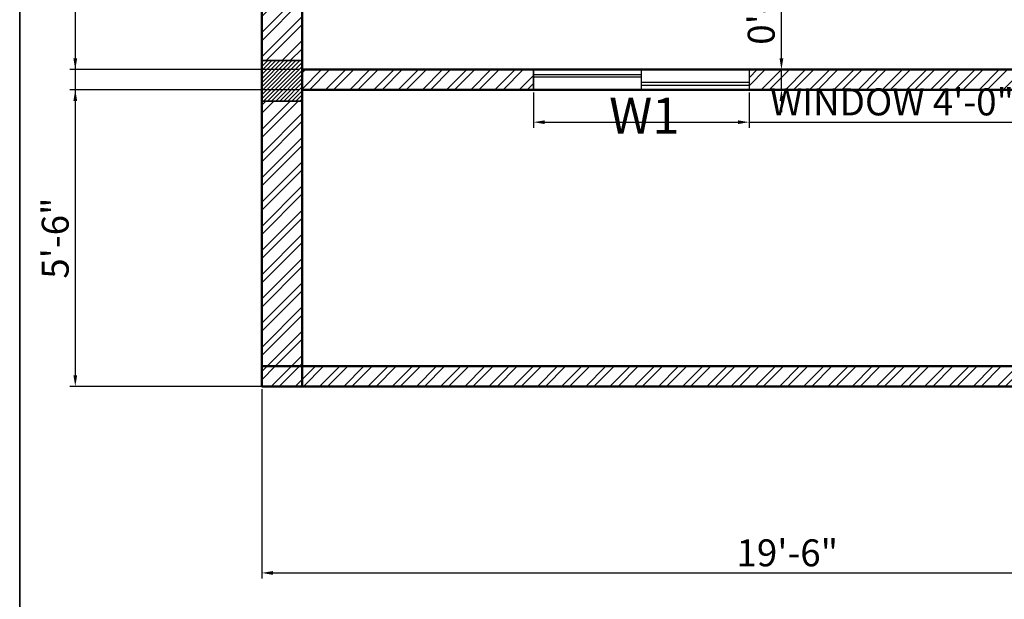
# Model space of a CAD drawing. Units: millimetres. Extents: x 20768 to 23556, y 50760 to 52704.
# Tile 15 of 36: x 21272 to 21491, y 51783 to 51912. Entities that reach past the tile are written whole.
import ezdxf

# ---------------------------------------------------------------- set-up
doc = ezdxf.new("R2010")
doc.units = ezdxf.units.MM
for name, color, linetype, lineweight in [('A-ANNO-TTLB', 7, 'Continuous', 35), ('A-AREA-IDEN', 40, 'Continuous', 18), ('A-GLAZ', 4, 'Continuous', 25), ('A-WALL', 7, 'Continuous', 50), ('A-WALL-PATT', 8, 'Continuous', 13), ('S-ANNO-DIMS', 2, 'Continuous', 18), ('S-COLS', 20, 'Continuous', 35)]:
    doc.layers.add(name, color=color, linetype=linetype, lineweight=lineweight)
doc.styles.get("Standard").update_dxf_attribs({"font": 'arial.ttf'})
doc.dimstyles.new('ISO-25', dxfattribs={"dimtxt": 6, "dimasz": 2.5, "dimexe": 1.25, "dimexo": 0.625, "dimtad": 1, "dimdec": 0, "dimlunit": 3, "dimtxsty": 'Standard', "dimcen": 2.5, "dimadec": 0, "dimazin": 0, "dimtfac": 1, "dimtdec": 0, "dimtmove": 0, "dimatfit": 3, "dimfxl": 1, "dimarcsym": 0})
pattern_1 = [(45, (-37.4434, 0), (-2.69407684, 2.69407684), []), (45, (-35.6473, 0), (-2.69407684, 2.69407684), [])]

# ---------------------------------------------------------------- blocks, each defined once
blk = doc.blocks.new('WIN-PLAN-C')
blk.add_line((0, 4.5), (0, 0))
blk.add_lwpolyline([(0, 4.5), (48, 4.5), (48, 0), (0, 0)], close=True)
blk = doc.blocks.new('*D179')
at = {"layer": 'Defpoints', "color": 0, "transparency": 16777216}
for p in [(21386.24, 51895.9), (21434.24, 51895.9), (21434.24, 51888.7)]:
    blk.add_point(p, dxfattribs=at)
at = {"layer": 'S-ANNO-DIMS', "color": 0, "lineweight": -2, "transparency": 16777216}
for p, q in [((21386.24, 51895.27), (21386.24, 51887.45)), ((21434.24, 51895.27), (21434.24, 51887.45)), ((21388.74, 51888.7), (21431.74, 51888.7)), ((21434.24, 51888.7), (21513.92, 51888.7))]:
    blk.add_line(p, q, dxfattribs=at)
at = {"layer": 'S-ANNO-DIMS', "color": 0, "transparency": 16777216}
for points in [[(21388.74, 51889.11), (21388.74, 51888.28), (21386.24, 51888.7)], [(21431.74, 51889.11), (21431.74, 51888.28), (21434.24, 51888.7)]]:
    blk.add_solid(points, dxfattribs=at)
at = {"layer": 'S-ANNO-DIMS', "color": 0, "transparency": 16777216, "insert": (21475.33, 51892.43), "char_height": 6, "attachment_point": 5}
blk.add_mtext('WINDOW 4\'-0" TYP.', dxfattribs=at)
blk = doc.blocks.new('*D180')
at = {"layer": 'Defpoints', "color": 0, "transparency": 16777216}
for p in [(21434.24, 51900.4), (21441.44, 51900.4), (21434.24, 51895.9)]:
    blk.add_point(p, dxfattribs=at)
at = {"layer": 'S-ANNO-DIMS', "color": 0, "lineweight": -2, "transparency": 16777216}
for p, q in [((21441.44, 51902.9), (21441.44, 51957.2)), ((21434.87, 51900.4), (21442.69, 51900.4)), ((21441.44, 51895.9), (21441.44, 51900.4)), ((21434.87, 51895.9), (21442.69, 51895.9)), ((21441.44, 51893.4), (21441.44, 51890.9))]:
    blk.add_line(p, q, dxfattribs=at)
at = {"layer": 'S-ANNO-DIMS', "color": 0, "transparency": 16777216}
for points in [[(21441.02, 51902.9), (21441.86, 51902.9), (21441.44, 51900.4)], [(21441.02, 51893.4), (21441.86, 51893.4), (21441.44, 51895.9)]]:
    blk.add_solid(points, dxfattribs=at)
at = {"layer": 'S-ANNO-DIMS', "color": 0, "transparency": 16777216, "insert": (21437.71, 51931.3), "char_height": 6, "attachment_point": 5, "rotation": 90}
blk.add_mtext('0\'-4 1/2" TYP.', dxfattribs=at)
blk = doc.blocks.new('*D210')
at = {"layer": 'Defpoints', "color": 0, "transparency": 16777216}
for p in [(21325.74, 51829.9), (21559.74, 51829.9), (21559.74, 51788.4)]:
    blk.add_point(p, dxfattribs=at)
at = {"layer": 'S-ANNO-DIMS', "color": 0, "lineweight": -2, "transparency": 16777216}
for p, q in [((21325.74, 51829.27), (21325.74, 51787.15)), ((21559.74, 51829.27), (21559.74, 51787.15)), ((21328.24, 51788.4), (21557.24, 51788.4))]:
    blk.add_line(p, q, dxfattribs=at)
at = {"layer": 'S-ANNO-DIMS', "color": 0, "transparency": 16777216}
for points in [[(21328.24, 51788.81), (21328.24, 51787.98), (21325.74, 51788.4)], [(21557.24, 51788.81), (21557.24, 51787.98), (21559.74, 51788.4)]]:
    blk.add_solid(points, dxfattribs=at)
at = {"layer": 'S-ANNO-DIMS', "color": 0, "transparency": 16777216, "insert": (21442.74, 51792.09), "char_height": 6, "attachment_point": 5}
blk.add_mtext('19\'-6"', dxfattribs=at)
blk = doc.blocks.new('*D211')
at = {"layer": 'Defpoints', "color": 0, "transparency": 16777216}
for p in [(21325.74, 52522.9), (21284.24, 51829.9), (21325.74, 51829.9)]:
    blk.add_point(p, dxfattribs=at)
at = {"layer": 'S-ANNO-DIMS', "color": 0, "lineweight": -2, "transparency": 16777216}
for p, q in [((21325.12, 52522.9), (21282.99, 52522.9)), ((21284.24, 52520.4), (21284.24, 51832.4)), ((21325.12, 51829.9), (21282.99, 51829.9))]:
    blk.add_line(p, q, dxfattribs=at)
at = {"layer": 'S-ANNO-DIMS', "color": 0, "transparency": 16777216}
for points in [[(21283.82, 52520.4), (21284.66, 52520.4), (21284.24, 52522.9)], [(21283.82, 51832.4), (21284.66, 51832.4), (21284.24, 51829.9)]]:
    blk.add_solid(points, dxfattribs=at)
at = {"layer": 'S-ANNO-DIMS', "color": 0, "transparency": 16777216, "insert": (21280.55, 52176.4), "char_height": 6, "attachment_point": 5, "rotation": 90}
blk.add_mtext('57\'-9"', dxfattribs=at)
blk = doc.blocks.new('*D212')
at = {"layer": 'Defpoints', "color": 0, "transparency": 16777216}
for p in [(21334.74, 52080.4), (21284.24, 51900.4), (21334.74, 51900.4)]:
    blk.add_point(p, dxfattribs=at)
at = {"layer": 'S-ANNO-DIMS', "color": 0, "lineweight": -2, "transparency": 16777216}
for p, q in [((21334.12, 52080.4), (21282.99, 52080.4)), ((21284.24, 52077.9), (21284.24, 51902.9)), ((21334.12, 51900.4), (21282.99, 51900.4))]:
    blk.add_line(p, q, dxfattribs=at)
at = {"layer": 'S-ANNO-DIMS', "color": 0, "transparency": 16777216}
for points in [[(21283.82, 52077.9), (21284.66, 52077.9), (21284.24, 52080.4)], [(21283.82, 51902.9), (21284.66, 51902.9), (21284.24, 51900.4)]]:
    blk.add_solid(points, dxfattribs=at)
at = {"layer": 'S-ANNO-DIMS', "color": 0, "transparency": 16777216, "insert": (21280.55, 51990.4), "char_height": 6, "attachment_point": 5, "rotation": 90}
blk.add_mtext('15\'-0"', dxfattribs=at)
blk = doc.blocks.new('*D213')
at = {"layer": 'Defpoints', "color": 0, "transparency": 16777216}
for p in [(21334.74, 51895.9), (21284.24, 51829.9), (21334.74, 51829.9)]:
    blk.add_point(p, dxfattribs=at)
at = {"layer": 'S-ANNO-DIMS', "color": 0, "lineweight": -2, "transparency": 16777216}
for p, q in [((21334.12, 51895.9), (21282.99, 51895.9)), ((21284.24, 51893.4), (21284.24, 51832.4)), ((21334.12, 51829.9), (21282.99, 51829.9))]:
    blk.add_line(p, q, dxfattribs=at)
at = {"layer": 'S-ANNO-DIMS', "color": 0, "transparency": 16777216}
for points in [[(21283.82, 51893.4), (21284.66, 51893.4), (21284.24, 51895.9)], [(21283.82, 51832.4), (21284.66, 51832.4), (21284.24, 51829.9)]]:
    blk.add_solid(points, dxfattribs=at)
at = {"layer": 'S-ANNO-DIMS', "color": 0, "transparency": 16777216, "insert": (21280.55, 51862.9), "char_height": 6, "attachment_point": 5, "rotation": 90}
blk.add_mtext('5\'-6"', dxfattribs=at)

msp = doc.modelspace()

# ---------------------------------------------------------------- hatches: boundary and pattern name
at = {"layer": 'A-WALL-PATT'}
h = msp.add_hatch(dxfattribs=at)
h.set_pattern_fill('ANSI32', color=256, scale=0.4)
h.set_pattern_definition(pattern_1)
h.paths.add_polyline_path([(21334.74, 52077.9), (21325.74, 52077.9), (21325.74, 51902.4), (21334.74, 51902.4)])
h = msp.add_hatch(dxfattribs=at)
h.set_pattern_fill('ANSI31', color=256, scale=0.2)
h.set_pattern_definition([(45, (345.4904, 0), (-0.449012806, 0.449012806), [])])
h.paths.add_polyline_path([(21334.74, 51902.4), (21325.74, 51902.4), (21325.74, 51893.4), (21334.74, 51893.4)])
h = msp.add_hatch(dxfattribs=at)
h.set_pattern_fill('ANSI32', color=256, scale=0.4)
h.set_pattern_definition(pattern_1)
h.paths.add_polyline_path([(21386.24, 51900.4), (21334.74, 51900.4), (21334.74, 51895.9), (21386.24, 51895.9)])
h = msp.add_hatch(dxfattribs=at)
h.set_pattern_fill('ANSI32', color=256, scale=0.4)
h.set_pattern_definition(pattern_1)
h.paths.add_polyline_path([(21507.24, 51898.42), (21507.24, 51900.4), (21434.24, 51900.4), (21434.24, 51895.9), (21507.24, 51895.9)])
h = msp.add_hatch(dxfattribs=at)
h.set_pattern_fill('ANSI32', color=256, scale=0.4)
h.set_pattern_definition(pattern_1)
h.paths.add_polyline_path([(21334.74, 51893.4), (21325.74, 51893.4), (21325.74, 51834.4), (21334.74, 51834.4)])
h = msp.add_hatch(dxfattribs=at)
h.set_pattern_fill('ANSI32', color=256, scale=0.4)
h.set_pattern_definition(pattern_1)
h.paths.add_polyline_path([(21559.74, 51893.4), (21550.74, 51893.4), (21550.74, 51834.4), (21334.74, 51834.4), (21334.74, 51829.9), (21559.74, 51829.9)])
h = msp.add_hatch(dxfattribs=at)
h.set_pattern_fill('ANSI32', color=256, scale=0.4)
h.set_pattern_definition(pattern_1)
h.paths.add_polyline_path([(21334.74, 51834.4), (21325.74, 51834.4), (21325.74, 51829.9), (21334.74, 51829.9)])

# ---------------------------------------------------------------- linework, layer by layer
at = {"layer": 'A-ANNO-TTLB'}
msp.add_line((21271.86, 52703.98), (21271.86, 51623.53), dxfattribs=at)
at = {"layer": 'A-GLAZ'}
for p, q in [((21410.24, 51900.4), (21410.24, 51895.9)), ((21434.24, 51900.4), (21434.24, 51895.9)), ((21410.24, 51899.26), (21386.24, 51899.26)), ((21410.24, 51898.69), (21386.24, 51898.69)), ((21410.24, 51897.57), (21434.24, 51897.57)), ((21410.24, 51896.96), (21434.24, 51896.96))]:
    msp.add_line(p, q, dxfattribs=at)
at = {"layer": 'A-WALL'}
for p, q in [((21325.74, 52522.9), (21325.74, 51829.9)), ((21334.74, 52513.9), (21334.74, 51829.9)), ((21334.74, 51900.4), (21507.24, 51900.4)), ((21334.74, 51895.9), (21507.24, 51895.9)), ((21325.74, 51834.4), (21550.74, 51834.4)), ((21325.74, 51829.9), (21559.74, 51829.9))]:
    msp.add_line(p, q, dxfattribs=at)
at = {"layer": 'S-COLS'}
msp.add_lwpolyline([(21334.74, 51902.4), (21325.74, 51902.4), (21325.74, 51893.4), (21334.74, 51893.4)], close=True, dxfattribs=at)

# ---------------------------------------------------------------- block references
at = {"layer": 'A-GLAZ'}
msp.add_blockref('WIN-PLAN-C', (21386.24, 51895.9), dxfattribs=at)

# ---------------------------------------------------------------- texts
at = {"layer": 'A-AREA-IDEN', "insert": (21403.09, 51894.15), "char_height": 8, "attachment_point": 1}
msp.add_mtext_dynamic_manual_height_columns('W1', width=27.5349, gutter_width=12.5, heights=[0], dxfattribs=at)

# ---------------------------------------------------------------- dimensions: what is measured, and where the dimension line sits
at = {"layer": 'S-ANNO-DIMS'}
for base, p1, p2, picture, middle in [((21284.24, 51829.9), (21325.74, 52522.9), (21325.74, 51829.9), '*D211', (21280.55, 52176.4)), ((21284.24, 51900.4), (21334.74, 52080.4), (21334.74, 51900.4), '*D212', (21280.55, 51990.4)), ((21284.24, 51829.9), (21334.74, 51895.9), (21334.74, 51829.9), '*D213', (21280.55, 51862.9))]:
    dim = msp.add_linear_dim(base=base, p1=p1, p2=p2, angle=90, dimstyle='ISO-25', override={"dimdec": 1, "dimlfac": 1, "dimrnd": 0, "dimzin": 1, "dimdsep": 46, "dimlunit": 4, "dimfrac": 2}, dxfattribs=at)
    dim.commit()
    dim.dimension.update_dxf_attribs({"geometry": picture, "text_midpoint": middle})
dim = msp.add_linear_dim(base=(21441.44, 51900.4), p1=(21434.24, 51895.9), p2=(21434.24, 51900.4), angle=90, text='<> TYP.', dimstyle='ISO-25', override={"dimdec": 1, "dimrnd": 0, "dimzin": 1, "dimlunit": 4, "dimfrac": 2}, dxfattribs=at)
dim.commit()
dim.dimension.update_dxf_attribs({"geometry": '*D180', "text_midpoint": (21437.71, 51931.3)})
dim = msp.add_linear_dim(base=(21434.24, 51888.7), p1=(21386.24, 51895.9), p2=(21434.24, 51895.9), text='WINDOW <> TYP.', dimstyle='ISO-25', override={"dimdec": 1, "dimrnd": 0, "dimzin": 1, "dimlunit": 4, "dimfrac": 2}, dxfattribs=at)
dim.commit()
dim.dimension.update_dxf_attribs({"geometry": '*D179', "text_midpoint": (21475.33, 51892.43)})
dim = msp.add_linear_dim(base=(21559.74, 51788.4), p1=(21325.74, 51829.9), p2=(21559.74, 51829.9), dimstyle='ISO-25', override={"dimdec": 1, "dimlfac": 1, "dimrnd": 0, "dimzin": 1, "dimdsep": 46, "dimlunit": 4, "dimfrac": 2}, dxfattribs=at)
dim.commit()
dim.dimension.update_dxf_attribs({"geometry": '*D210', "text_midpoint": (21442.74, 51792.09)})

doc.saveas('drawing.dxf')
